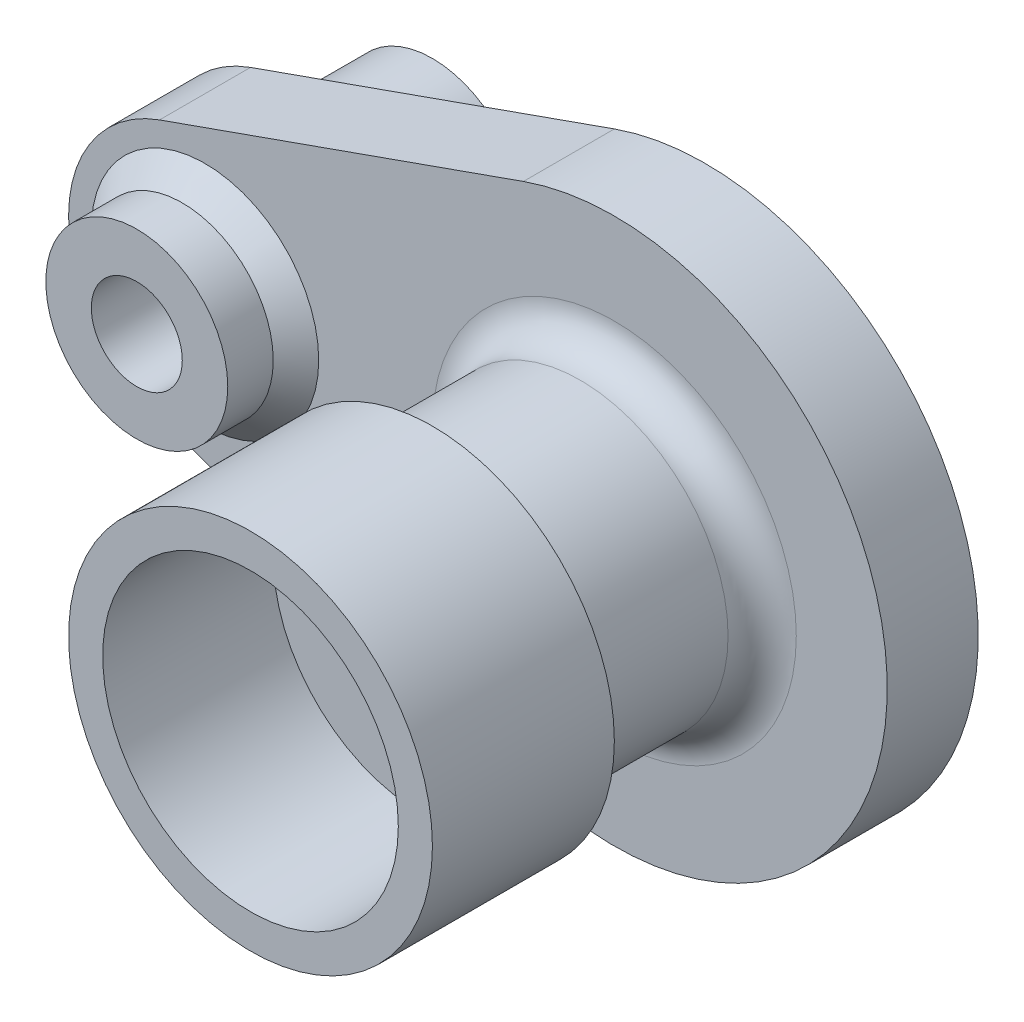
ISO-10303-21;
HEADER;
FILE_DESCRIPTION(('STEP AP214'),'2;1');
FILE_NAME('part.step','',(''),(''),'','','');
FILE_SCHEMA(('AUTOMOTIVE_DESIGN { 1 0 10303 214 1 1 1 1 }'));
ENDSEC;
DATA;
#1=APPLICATION_CONTEXT('core data for automotive mechanical design processes');
#2=APPLICATION_PROTOCOL_DEFINITION('international standard','automotive_design',2000,#1);
#3=PRODUCT_CONTEXT('',#1,'mechanical');
#4=PRODUCT('Part','Part','',(#3));
#5=PRODUCT_RELATED_PRODUCT_CATEGORY('part','',(#4));
#6=PRODUCT_DEFINITION_FORMATION('','',#4);
#7=PRODUCT_DEFINITION_CONTEXT('part definition',#1,'design');
#8=PRODUCT_DEFINITION('design','',#6,#7);
#9=PRODUCT_DEFINITION_SHAPE('','',#8);
#10=(LENGTH_UNIT() NAMED_UNIT(*) SI_UNIT(.MILLI.,.METRE.));
#11=(NAMED_UNIT(*) PLANE_ANGLE_UNIT() SI_UNIT($,.RADIAN.));
#12=(NAMED_UNIT(*) SI_UNIT($,.STERADIAN.) SOLID_ANGLE_UNIT());
#13=UNCERTAINTY_MEASURE_WITH_UNIT(LENGTH_MEASURE(1.E-05),#10,'distance_accuracy_value','');
#14=(GEOMETRIC_REPRESENTATION_CONTEXT(3) GLOBAL_UNCERTAINTY_ASSIGNED_CONTEXT((#13)) GLOBAL_UNIT_ASSIGNED_CONTEXT((#10,
#11,#12)) REPRESENTATION_CONTEXT('',''));
#15=CARTESIAN_POINT('',(0.,0.,0.));
#16=DIRECTION('',(0.,0.,1.));
#17=DIRECTION('',(1.,0.,0.));
#18=AXIS2_PLACEMENT_3D('',#15,#16,#17);
#19=CARTESIAN_POINT('',(-8.00000000000001,22.6274169979695,8.));
#20=DIRECTION('',(-0.333333333333333,0.942809041582063,0.));
#21=DIRECTION('',(-0.942809041582063,-0.333333333333334,0.));
#22=AXIS2_PLACEMENT_3D('',#19,#20,#21);
#23=PLANE('',#22);
#24=DIRECTION('',(0.942809041582063,0.333333333333334,0.));
#25=VECTOR('',#24,1.);
#26=CARTESIAN_POINT('',(-8.00000000000001,22.6274169979695,0.));
#27=LINE('',#26,#25);
#28=CARTESIAN_POINT('',(-40.,11.3137084989848,0.));
#29=VERTEX_POINT('',#28);
#30=CARTESIAN_POINT('',(-8.00000000000001,22.6274169979695,0.));
#31=VERTEX_POINT('',#30);
#32=EDGE_CURVE('E118',#29,#31,#27,.T.);
#33=ORIENTED_EDGE('',*,*,#32,.F.);
#34=DIRECTION('',(0.,0.,-1.));
#35=VECTOR('',#34,1.);
#36=CARTESIAN_POINT('',(-40.,11.3137084989848,8.));
#37=LINE('',#36,#35);
#38=CARTESIAN_POINT('',(-40.,11.3137084989848,8.));
#39=VERTEX_POINT('',#38);
#40=EDGE_CURVE('E94',#39,#29,#37,.T.);
#41=ORIENTED_EDGE('',*,*,#40,.F.);
#42=DIRECTION('',(0.942809041582063,0.333333333333334,0.));
#43=VECTOR('',#42,1.);
#44=CARTESIAN_POINT('',(-8.00000000000001,22.6274169979695,8.));
#45=LINE('',#44,#43);
#46=CARTESIAN_POINT('',(-8.00000000000001,22.6274169979695,8.));
#47=VERTEX_POINT('',#46);
#48=EDGE_CURVE('E105',#39,#47,#45,.T.);
#49=ORIENTED_EDGE('',*,*,#48,.T.);
#50=DIRECTION('',(0.,0.,-1.));
#51=VECTOR('',#50,1.);
#52=CARTESIAN_POINT('',(-8.00000000000001,22.6274169979695,8.));
#53=LINE('',#52,#51);
#54=EDGE_CURVE('E89',#47,#31,#53,.T.);
#55=ORIENTED_EDGE('',*,*,#54,.T.);
#56=EDGE_LOOP('',(#33,#41,#49,#55));
#57=FACE_BOUND('',#56,.T.);
#58=ADVANCED_FACE('F50',(#57),#23,.T.);
#59=CARTESIAN_POINT('',(-36.,0.,8.));
#60=DIRECTION('',(0.,0.,-1.));
#61=DIRECTION('',(-1.,0.,0.));
#62=AXIS2_PLACEMENT_3D('',#59,#60,#61);
#63=CYLINDRICAL_SURFACE('',#62,12.);
#64=CARTESIAN_POINT('',(-36.,0.,0.));
#65=DIRECTION('',(0.,0.,1.));
#66=DIRECTION('',(1.,0.,0.));
#67=AXIS2_PLACEMENT_3D('',#64,#65,#66);
#68=CIRCLE('',#67,12.);
#69=CARTESIAN_POINT('',(-40.,-11.3137084989848,0.));
#70=VERTEX_POINT('',#69);
#71=EDGE_CURVE('E107',#29,#70,#68,.T.);
#72=ORIENTED_EDGE('',*,*,#71,.T.);
#73=DIRECTION('',(0.,0.,-1.));
#74=VECTOR('',#73,1.);
#75=CARTESIAN_POINT('',(-40.,-11.3137084989848,8.));
#76=LINE('',#75,#74);
#77=CARTESIAN_POINT('',(-40.,-11.3137084989848,8.));
#78=VERTEX_POINT('',#77);
#79=EDGE_CURVE('E104',#78,#70,#76,.T.);
#80=ORIENTED_EDGE('',*,*,#79,.F.);
#81=CARTESIAN_POINT('',(-36.,0.,8.));
#82=DIRECTION('',(0.,0.,1.));
#83=DIRECTION('',(1.,0.,0.));
#84=AXIS2_PLACEMENT_3D('',#81,#82,#83);
#85=CIRCLE('',#84,12.);
#86=EDGE_CURVE('E100',#39,#78,#85,.T.);
#87=ORIENTED_EDGE('',*,*,#86,.F.);
#88=ORIENTED_EDGE('',*,*,#40,.T.);
#89=EDGE_LOOP('',(#72,#80,#87,#88));
#90=FACE_BOUND('',#89,.T.);
#91=ADVANCED_FACE('F106',(#90),#63,.T.);
#92=CARTESIAN_POINT('',(-8.,-22.6274169979695,8.));
#93=DIRECTION('',(0.333333333333333,0.942809041582063,0.));
#94=DIRECTION('',(-0.942809041582063,0.333333333333333,0.));
#95=AXIS2_PLACEMENT_3D('',#92,#93,#94);
#96=PLANE('',#95);
#97=DIRECTION('',(0.942809041582063,-0.333333333333333,0.));
#98=VECTOR('',#97,1.);
#99=CARTESIAN_POINT('',(-8.,-22.6274169979695,0.));
#100=LINE('',#99,#98);
#101=CARTESIAN_POINT('',(-8.,-22.6274169979695,0.));
#102=VERTEX_POINT('',#101);
#103=EDGE_CURVE('E81',#70,#102,#100,.T.);
#104=ORIENTED_EDGE('',*,*,#103,.T.);
#105=DIRECTION('',(0.,0.,-1.));
#106=VECTOR('',#105,1.);
#107=CARTESIAN_POINT('',(-8.,-22.6274169979695,8.));
#108=LINE('',#107,#106);
#109=CARTESIAN_POINT('',(-8.,-22.6274169979695,8.));
#110=VERTEX_POINT('',#109);
#111=EDGE_CURVE('E108',#110,#102,#108,.T.);
#112=ORIENTED_EDGE('',*,*,#111,.F.);
#113=DIRECTION('',(0.942809041582063,-0.333333333333333,0.));
#114=VECTOR('',#113,1.);
#115=CARTESIAN_POINT('',(-8.,-22.6274169979695,8.));
#116=LINE('',#115,#114);
#117=EDGE_CURVE('E101',#78,#110,#116,.T.);
#118=ORIENTED_EDGE('',*,*,#117,.F.);
#119=ORIENTED_EDGE('',*,*,#79,.T.);
#120=EDGE_LOOP('',(#104,#112,#118,#119));
#121=FACE_BOUND('',#120,.T.);
#122=ADVANCED_FACE('F112',(#121),#96,.F.);
#123=CARTESIAN_POINT('',(0.,0.,8.));
#124=DIRECTION('',(0.,0.,-1.));
#125=DIRECTION('',(-1.,0.,0.));
#126=AXIS2_PLACEMENT_3D('',#123,#124,#125);
#127=CYLINDRICAL_SURFACE('',#126,24.);
#128=CARTESIAN_POINT('',(0.,0.,0.));
#129=DIRECTION('',(0.,0.,1.));
#130=DIRECTION('',(1.,0.,0.));
#131=AXIS2_PLACEMENT_3D('',#128,#129,#130);
#132=CIRCLE('',#131,24.);
#133=EDGE_CURVE('E125',#102,#31,#132,.T.);
#134=ORIENTED_EDGE('',*,*,#133,.T.);
#135=ORIENTED_EDGE('',*,*,#54,.F.);
#136=CARTESIAN_POINT('',(0.,0.,8.));
#137=DIRECTION('',(0.,0.,1.));
#138=DIRECTION('',(1.,0.,0.));
#139=AXIS2_PLACEMENT_3D('',#136,#137,#138);
#140=CIRCLE('',#139,24.);
#141=EDGE_CURVE('E68',#110,#47,#140,.T.);
#142=ORIENTED_EDGE('',*,*,#141,.F.);
#143=ORIENTED_EDGE('',*,*,#111,.T.);
#144=EDGE_LOOP('',(#134,#135,#142,#143));
#145=FACE_BOUND('',#144,.T.);
#146=ADVANCED_FACE('F163',(#145),#127,.T.);
#147=CARTESIAN_POINT('',(0.,0.,8.));
#148=DIRECTION('',(0.,0.,1.));
#149=DIRECTION('',(1.,0.,0.));
#150=AXIS2_PLACEMENT_3D('',#147,#148,#149);
#151=PLANE('',#150);
#152=CARTESIAN_POINT('',(-36.,0.,8.));
#153=DIRECTION('',(0.,0.,1.));
#154=DIRECTION('',(1.,0.,0.));
#155=AXIS2_PLACEMENT_3D('',#152,#153,#154);
#156=CIRCLE('',#155,9.99999999999999);
#157=CARTESIAN_POINT('',(-26.,0.,8.));
#158=VERTEX_POINT('',#157);
#159=EDGE_CURVE('E11',#158,#158,#156,.F.);
#160=ORIENTED_EDGE('',*,*,#159,.T.);
#161=EDGE_LOOP('',(#160));
#162=FACE_BOUND('',#161,.T.);
#163=CARTESIAN_POINT('',(0.,0.,8.));
#164=DIRECTION('',(0.,0.,1.));
#165=DIRECTION('',(1.,0.,0.));
#166=AXIS2_PLACEMENT_3D('',#163,#164,#165);
#167=CIRCLE('',#166,16.);
#168=CARTESIAN_POINT('',(16.,0.,8.));
#169=VERTEX_POINT('',#168);
#170=EDGE_CURVE('E131',#169,#169,#167,.F.);
#171=ORIENTED_EDGE('',*,*,#170,.T.);
#172=EDGE_LOOP('',(#171));
#173=FACE_BOUND('',#172,.T.);
#174=ORIENTED_EDGE('',*,*,#48,.F.);
#175=ORIENTED_EDGE('',*,*,#86,.T.);
#176=ORIENTED_EDGE('',*,*,#117,.T.);
#177=ORIENTED_EDGE('',*,*,#141,.T.);
#178=EDGE_LOOP('',(#174,#175,#176,#177));
#179=FACE_BOUND('',#178,.T.);
#180=ADVANCED_FACE('F97',(#162,#173,#179),#151,.T.);
#181=CARTESIAN_POINT('',(0.,0.,0.));
#182=DIRECTION('',(0.,0.,1.));
#183=DIRECTION('',(1.,0.,0.));
#184=AXIS2_PLACEMENT_3D('',#181,#182,#183);
#185=PLANE('',#184);
#186=CARTESIAN_POINT('',(-36.,0.,0.));
#187=DIRECTION('',(0.,0.,1.));
#188=DIRECTION('',(1.,0.,0.));
#189=AXIS2_PLACEMENT_3D('',#186,#187,#188);
#190=CIRCLE('',#189,8.);
#191=CARTESIAN_POINT('',(-28.,0.,0.));
#192=VERTEX_POINT('',#191);
#193=EDGE_CURVE('E130',#192,#192,#190,.F.);
#194=ORIENTED_EDGE('',*,*,#193,.F.);
#195=EDGE_LOOP('',(#194));
#196=FACE_BOUND('',#195,.T.);
#197=ORIENTED_EDGE('',*,*,#32,.T.);
#198=ORIENTED_EDGE('',*,*,#133,.F.);
#199=ORIENTED_EDGE('',*,*,#103,.F.);
#200=ORIENTED_EDGE('',*,*,#71,.F.);
#201=EDGE_LOOP('',(#197,#198,#199,#200));
#202=FACE_BOUND('',#201,.T.);
#203=ADVANCED_FACE('F169',(#196,#202),#185,.F.);
#204=CARTESIAN_POINT('',(-36.,0.,14.));
#205=DIRECTION('',(0.,0.,-1.));
#206=DIRECTION('',(-1.,0.,0.));
#207=AXIS2_PLACEMENT_3D('',#204,#205,#206);
#208=CYLINDRICAL_SURFACE('',#207,8.);
#209=CARTESIAN_POINT('',(-36.,0.,10.));
#210=DIRECTION('',(0.,0.,1.));
#211=DIRECTION('',(1.,0.,0.));
#212=AXIS2_PLACEMENT_3D('',#209,#210,#211);
#213=CIRCLE('',#212,8.);
#214=CARTESIAN_POINT('',(-28.,0.,10.));
#215=VERTEX_POINT('',#214);
#216=EDGE_CURVE('E59',#215,#215,#213,.T.);
#217=ORIENTED_EDGE('',*,*,#216,.T.);
#218=EDGE_LOOP('',(#217));
#219=FACE_BOUND('',#218,.T.);
#220=CARTESIAN_POINT('',(-36.,0.,14.));
#221=DIRECTION('',(0.,0.,1.));
#222=DIRECTION('',(1.,0.,0.));
#223=AXIS2_PLACEMENT_3D('',#220,#221,#222);
#224=CIRCLE('',#223,8.);
#225=CARTESIAN_POINT('',(-28.,0.,14.));
#226=VERTEX_POINT('',#225);
#227=EDGE_CURVE('E119',#226,#226,#224,.T.);
#228=ORIENTED_EDGE('',*,*,#227,.F.);
#229=EDGE_LOOP('',(#228));
#230=FACE_BOUND('',#229,.T.);
#231=ADVANCED_FACE('F137',(#219,#230),#208,.T.);
#232=CARTESIAN_POINT('',(-36.,0.,14.));
#233=DIRECTION('',(0.,0.,1.));
#234=DIRECTION('',(1.,0.,0.));
#235=AXIS2_PLACEMENT_3D('',#232,#233,#234);
#236=PLANE('',#235);
#237=CARTESIAN_POINT('',(-36.,0.,14.));
#238=DIRECTION('',(0.,0.,1.));
#239=DIRECTION('',(1.,0.,0.));
#240=AXIS2_PLACEMENT_3D('',#237,#238,#239);
#241=CIRCLE('',#240,4.);
#242=CARTESIAN_POINT('',(-32.,0.,14.));
#243=VERTEX_POINT('',#242);
#244=EDGE_CURVE('E223',#243,#243,#241,.T.);
#245=ORIENTED_EDGE('',*,*,#244,.F.);
#246=EDGE_LOOP('',(#245));
#247=FACE_BOUND('',#246,.T.);
#248=ORIENTED_EDGE('',*,*,#227,.T.);
#249=EDGE_LOOP('',(#248));
#250=FACE_BOUND('',#249,.T.);
#251=ADVANCED_FACE('F180',(#247,#250),#236,.T.);
#252=CARTESIAN_POINT('',(-36.,0.,-12.));
#253=DIRECTION('',(0.,0.,1.));
#254=DIRECTION('',(1.,0.,0.));
#255=AXIS2_PLACEMENT_3D('',#252,#253,#254);
#256=CYLINDRICAL_SURFACE('',#255,8.);
#257=CARTESIAN_POINT('',(-36.,0.,-12.));
#258=DIRECTION('',(0.,0.,-1.));
#259=DIRECTION('',(-1.,0.,0.));
#260=AXIS2_PLACEMENT_3D('',#257,#258,#259);
#261=CIRCLE('',#260,8.);
#262=CARTESIAN_POINT('',(-44.,0.,-12.));
#263=VERTEX_POINT('',#262);
#264=EDGE_CURVE('E235',#263,#263,#261,.T.);
#265=ORIENTED_EDGE('',*,*,#264,.F.);
#266=EDGE_LOOP('',(#265));
#267=FACE_BOUND('',#266,.T.);
#268=ORIENTED_EDGE('',*,*,#193,.T.);
#269=EDGE_LOOP('',(#268));
#270=FACE_BOUND('',#269,.T.);
#271=ADVANCED_FACE('F179',(#267,#270),#256,.T.);
#272=CARTESIAN_POINT('',(-36.,0.,-12.));
#273=DIRECTION('',(0.,0.,-1.));
#274=DIRECTION('',(-1.,0.,0.));
#275=AXIS2_PLACEMENT_3D('',#272,#273,#274);
#276=PLANE('',#275);
#277=CARTESIAN_POINT('',(-36.,0.,-12.));
#278=DIRECTION('',(0.,0.,-1.));
#279=DIRECTION('',(-1.,0.,0.));
#280=AXIS2_PLACEMENT_3D('',#277,#278,#279);
#281=CIRCLE('',#280,4.);
#282=CARTESIAN_POINT('',(-40.,0.,-12.));
#283=VERTEX_POINT('',#282);
#284=EDGE_CURVE('E55',#283,#283,#281,.T.);
#285=ORIENTED_EDGE('',*,*,#284,.F.);
#286=EDGE_LOOP('',(#285));
#287=FACE_BOUND('',#286,.T.);
#288=ORIENTED_EDGE('',*,*,#264,.T.);
#289=EDGE_LOOP('',(#288));
#290=FACE_BOUND('',#289,.T.);
#291=ADVANCED_FACE('F184',(#287,#290),#276,.T.);
#292=CARTESIAN_POINT('',(0.,0.,24.));
#293=DIRECTION('',(0.,0.,-1.));
#294=DIRECTION('',(-1.,0.,0.));
#295=AXIS2_PLACEMENT_3D('',#292,#293,#294);
#296=CYLINDRICAL_SURFACE('',#295,13.);
#297=CARTESIAN_POINT('',(0.,0.,11.));
#298=DIRECTION('',(0.,0.,1.));
#299=DIRECTION('',(1.,0.,0.));
#300=AXIS2_PLACEMENT_3D('',#297,#298,#299);
#301=CIRCLE('',#300,13.);
#302=CARTESIAN_POINT('',(13.,0.,11.));
#303=VERTEX_POINT('',#302);
#304=EDGE_CURVE('E128',#303,#303,#301,.T.);
#305=ORIENTED_EDGE('',*,*,#304,.T.);
#306=EDGE_LOOP('',(#305));
#307=FACE_BOUND('',#306,.T.);
#308=CARTESIAN_POINT('',(0.,0.,24.));
#309=DIRECTION('',(0.,0.,1.));
#310=DIRECTION('',(1.,0.,0.));
#311=AXIS2_PLACEMENT_3D('',#308,#309,#310);
#312=CIRCLE('',#311,13.);
#313=CARTESIAN_POINT('',(13.,0.,24.));
#314=VERTEX_POINT('',#313);
#315=EDGE_CURVE('E226',#314,#314,#312,.T.);
#316=ORIENTED_EDGE('',*,*,#315,.F.);
#317=EDGE_LOOP('',(#316));
#318=FACE_BOUND('',#317,.T.);
#319=ADVANCED_FACE('F186',(#307,#318),#296,.T.);
#320=CARTESIAN_POINT('',(0.,0.,40.));
#321=DIRECTION('',(0.,0.,-1.));
#322=DIRECTION('',(-1.,0.,0.));
#323=AXIS2_PLACEMENT_3D('',#320,#321,#322);
#324=CYLINDRICAL_SURFACE('',#323,16.);
#325=CARTESIAN_POINT('',(0.,0.,40.));
#326=DIRECTION('',(0.,0.,1.));
#327=DIRECTION('',(1.,0.,0.));
#328=AXIS2_PLACEMENT_3D('',#325,#326,#327);
#329=CIRCLE('',#328,16.);
#330=CARTESIAN_POINT('',(16.,0.,40.));
#331=VERTEX_POINT('',#330);
#332=EDGE_CURVE('E219',#331,#331,#329,.T.);
#333=ORIENTED_EDGE('',*,*,#332,.F.);
#334=EDGE_LOOP('',(#333));
#335=FACE_BOUND('',#334,.T.);
#336=CARTESIAN_POINT('',(0.,0.,24.));
#337=DIRECTION('',(0.,0.,1.));
#338=DIRECTION('',(1.,0.,0.));
#339=AXIS2_PLACEMENT_3D('',#336,#337,#338);
#340=CIRCLE('',#339,16.);
#341=CARTESIAN_POINT('',(16.,0.,24.));
#342=VERTEX_POINT('',#341);
#343=EDGE_CURVE('E216',#342,#342,#340,.T.);
#344=ORIENTED_EDGE('',*,*,#343,.T.);
#345=EDGE_LOOP('',(#344));
#346=FACE_BOUND('',#345,.T.);
#347=ADVANCED_FACE('F195',(#335,#346),#324,.T.);
#348=CARTESIAN_POINT('',(0.,0.,40.));
#349=DIRECTION('',(0.,0.,1.));
#350=DIRECTION('',(1.,0.,0.));
#351=AXIS2_PLACEMENT_3D('',#348,#349,#350);
#352=PLANE('',#351);
#353=CARTESIAN_POINT('',(0.,0.,40.));
#354=DIRECTION('',(0.,0.,1.));
#355=DIRECTION('',(1.,0.,0.));
#356=AXIS2_PLACEMENT_3D('',#353,#354,#355);
#357=CIRCLE('',#356,13.);
#358=CARTESIAN_POINT('',(13.,0.,40.));
#359=VERTEX_POINT('',#358);
#360=EDGE_CURVE('E220',#359,#359,#357,.T.);
#361=ORIENTED_EDGE('',*,*,#360,.F.);
#362=EDGE_LOOP('',(#361));
#363=FACE_BOUND('',#362,.T.);
#364=ORIENTED_EDGE('',*,*,#332,.T.);
#365=EDGE_LOOP('',(#364));
#366=FACE_BOUND('',#365,.T.);
#367=ADVANCED_FACE('F198',(#363,#366),#352,.T.);
#368=CARTESIAN_POINT('',(0.,0.,24.));
#369=DIRECTION('',(0.,0.,1.));
#370=DIRECTION('',(1.,0.,0.));
#371=AXIS2_PLACEMENT_3D('',#368,#369,#370);
#372=PLANE('',#371);
#373=ORIENTED_EDGE('',*,*,#315,.T.);
#374=EDGE_LOOP('',(#373));
#375=FACE_BOUND('',#374,.T.);
#376=ORIENTED_EDGE('',*,*,#343,.F.);
#377=EDGE_LOOP('',(#376));
#378=FACE_BOUND('',#377,.T.);
#379=ADVANCED_FACE('F196',(#375,#378),#372,.F.);
#380=CARTESIAN_POINT('',(0.,0.,25.));
#381=DIRECTION('',(0.,0.,1.));
#382=DIRECTION('',(1.,0.,0.));
#383=AXIS2_PLACEMENT_3D('',#380,#381,#382);
#384=CYLINDRICAL_SURFACE('',#383,13.);
#385=CARTESIAN_POINT('',(0.,0.,25.));
#386=DIRECTION('',(0.,0.,1.));
#387=DIRECTION('',(1.,0.,0.));
#388=AXIS2_PLACEMENT_3D('',#385,#386,#387);
#389=CIRCLE('',#388,13.);
#390=CARTESIAN_POINT('',(13.,0.,25.));
#391=VERTEX_POINT('',#390);
#392=EDGE_CURVE('E214',#391,#391,#389,.T.);
#393=ORIENTED_EDGE('',*,*,#392,.F.);
#394=EDGE_LOOP('',(#393));
#395=FACE_BOUND('',#394,.T.);
#396=ORIENTED_EDGE('',*,*,#360,.T.);
#397=EDGE_LOOP('',(#396));
#398=FACE_BOUND('',#397,.T.);
#399=ADVANCED_FACE('F203',(#395,#398),#384,.F.);
#400=CARTESIAN_POINT('',(0.,0.,25.));
#401=DIRECTION('',(0.,0.,1.));
#402=DIRECTION('',(1.,0.,0.));
#403=AXIS2_PLACEMENT_3D('',#400,#401,#402);
#404=PLANE('',#403);
#405=ORIENTED_EDGE('',*,*,#392,.T.);
#406=EDGE_LOOP('',(#405));
#407=FACE_BOUND('',#406,.T.);
#408=ADVANCED_FACE('F155',(#407),#404,.T.);
#409=CARTESIAN_POINT('',(0.,0.,11.));
#410=DIRECTION('',(0.,0.,1.));
#411=DIRECTION('',(1.,0.,0.));
#412=AXIS2_PLACEMENT_3D('',#409,#410,#411);
#413=TOROIDAL_SURFACE('',#412,16.,3.);
#414=ORIENTED_EDGE('',*,*,#170,.F.);
#415=EDGE_LOOP('',(#414));
#416=FACE_BOUND('',#415,.T.);
#417=ORIENTED_EDGE('',*,*,#304,.F.);
#418=EDGE_LOOP('',(#417));
#419=FACE_BOUND('',#418,.T.);
#420=ADVANCED_FACE('F145',(#416,#419),#413,.F.);
#421=CARTESIAN_POINT('',(-36.,0.,10.));
#422=DIRECTION('',(0.,0.,-1.));
#423=DIRECTION('',(-1.,0.,0.));
#424=AXIS2_PLACEMENT_3D('',#421,#422,#423);
#425=CONICAL_SURFACE('',#424,8.,0.785398163397445);
#426=ORIENTED_EDGE('',*,*,#159,.F.);
#427=EDGE_LOOP('',(#426));
#428=FACE_BOUND('',#427,.T.);
#429=ORIENTED_EDGE('',*,*,#216,.F.);
#430=EDGE_LOOP('',(#429));
#431=FACE_BOUND('',#430,.T.);
#432=ADVANCED_FACE('F49',(#428,#431),#425,.T.);
#433=CARTESIAN_POINT('',(-36.,0.,-36.));
#434=DIRECTION('',(0.,0.,1.));
#435=DIRECTION('',(1.,0.,0.));
#436=AXIS2_PLACEMENT_3D('',#433,#434,#435);
#437=CYLINDRICAL_SURFACE('',#436,4.);
#438=ORIENTED_EDGE('',*,*,#284,.T.);
#439=EDGE_LOOP('',(#438));
#440=FACE_BOUND('',#439,.T.);
#441=ORIENTED_EDGE('',*,*,#244,.T.);
#442=EDGE_LOOP('',(#441));
#443=FACE_BOUND('',#442,.T.);
#444=ADVANCED_FACE('F141',(#440,#443),#437,.F.);
#445=CLOSED_SHELL('',(#58,#91,#122,#146,#180,#203,#231,#251,#271,#291,#319,#347,#367,#379,#399,
#408,#420,#432,#444));
#446=MANIFOLD_SOLID_BREP('B2',#445);
#447=ADVANCED_BREP_SHAPE_REPRESENTATION('',(#18,#446),#14);
#448=SHAPE_DEFINITION_REPRESENTATION(#9,#447);
ENDSEC;
END-ISO-10303-21;
